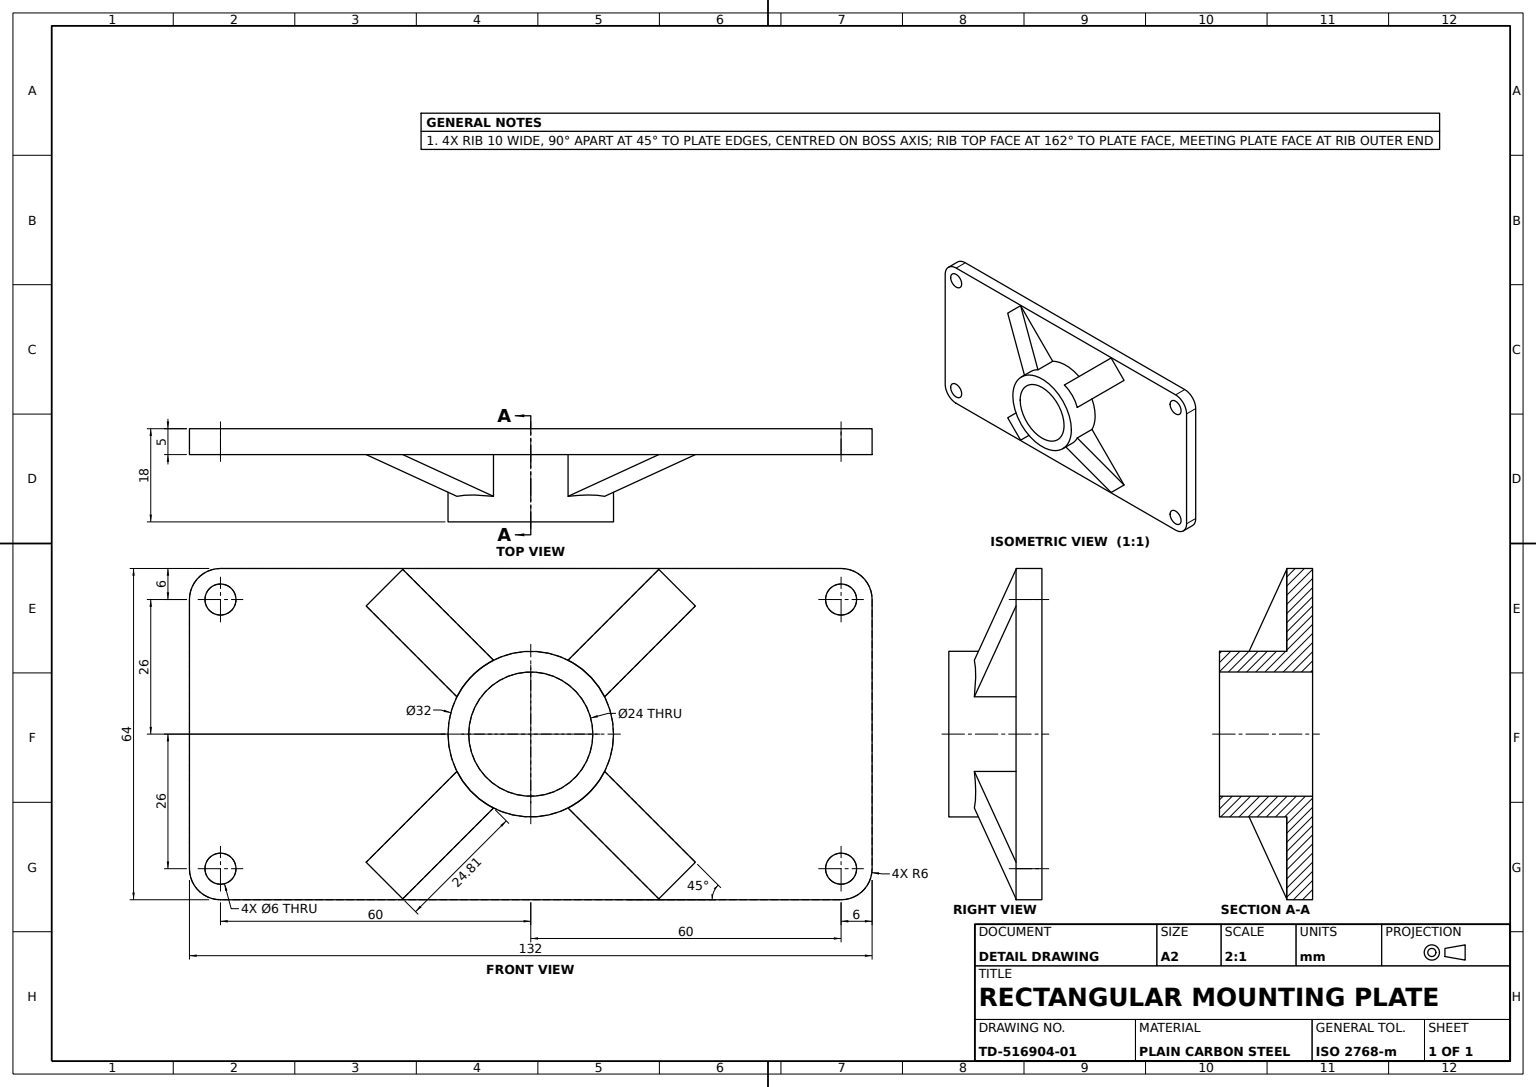
from build123d import *

# Parameters (mm, degrees)
PLATE_PROFILE_R           = 3
PLATE_PROFILE_R_2         = 12
BASE_PLATE_132X64X5_DEPTH = 5
HUB_PROFILE_R             = 16
HUB_PROFILE_R_2           = 12
HUB_BOSS_DEPTH            = 13
HUB_RIB_10MM_REACH        = 77.525
RIB_PROFILE_WALL_W        = 198.049660708
RIB_PROFILE_WALL_H        = 10
RIB_PATTERN_4X_COUNT      = 4


with BuildPart() as part:
    # Plate Profile → Base Plate 132x64x5 (new body)
    with BuildSketch(Plane.XY):
        with BuildLine():
            Line((-60, -32), (60, -32))
            ThreePointArc((60, -32), (64.242640687, -30.242640687), (66, -26))
            Line((66, -26), (66, 26))
            ThreePointArc((66, 26), (64.242640687, 30.242640687), (60, 32))
            Line((60, 32), (-60, 32))
            ThreePointArc((-60, 32), (-64.242640687, 30.242640687), (-66, 26))
            Line((-66, 26), (-66, -26))
            ThreePointArc((-66, -26), (-64.242640687, -30.242640687), (-60, -32))
        make_face()
        with Locations((-60, 26)):
            Circle(PLATE_PROFILE_R, mode=Mode.SUBTRACT)
        with Locations((60, 26)):
            Circle(PLATE_PROFILE_R, mode=Mode.SUBTRACT)
        with Locations((60, -26)):
            Circle(PLATE_PROFILE_R, mode=Mode.SUBTRACT)
        with Locations((-60, -26)):
            Circle(PLATE_PROFILE_R, mode=Mode.SUBTRACT)
        Circle(PLATE_PROFILE_R_2, mode=Mode.SUBTRACT)
    extrude(amount=BASE_PLATE_132X64X5_DEPTH)

    # Hub Profile → Hub Boss (add)
    with BuildSketch(Plane.XY.offset(5)):
        with Locations(Location((0, 0, 0), (0, 0, 180))):
            Circle(HUB_PROFILE_R)
        Circle(HUB_PROFILE_R_2, mode=Mode.SUBTRACT)
    extrude(amount=HUB_BOSS_DEPTH)

    # Rib Profile wall → Hub Rib 10mm (add, up to next)
    with BuildSketch(Plane(origin=(-15.131216519, -15.131216519, 11.047117627), x_dir=(-0.672498511963, -0.672498511963, -0.309016994381), z_dir=(-0.218508012229, -0.218508012229, 0.951056516293)), mode=Mode.PRIVATE) as hub_rib_10mm_sk1:
        Rectangle(RIB_PROFILE_WALL_W, RIB_PROFILE_WALL_H)
    hub_rib_10mm_tool1 = extrude(hub_rib_10mm_sk1.sketch, amount=-HUB_RIB_10MM_REACH, mode=Mode.PRIVATE) - part.part
    hub_rib_10mm = hub_rib_10mm_tool1.solids().sort_by_distance((-15.131216519, -15.131216519, 11.047117627))[0]
    add(hub_rib_10mm)

    # Rib Pattern 4x: Hub Rib 10mm ×4 about axis
    rib_pattern_4x_axis = Axis((0, 0, 0), (0, 0, 1))
    for i in range(1, RIB_PATTERN_4X_COUNT):
        add(hub_rib_10mm.rotate(rib_pattern_4x_axis, i * 360 / RIB_PATTERN_4X_COUNT))


solid = part.part
